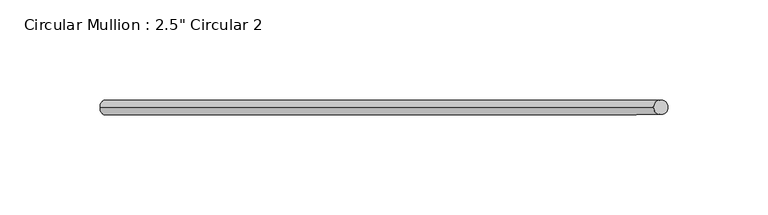
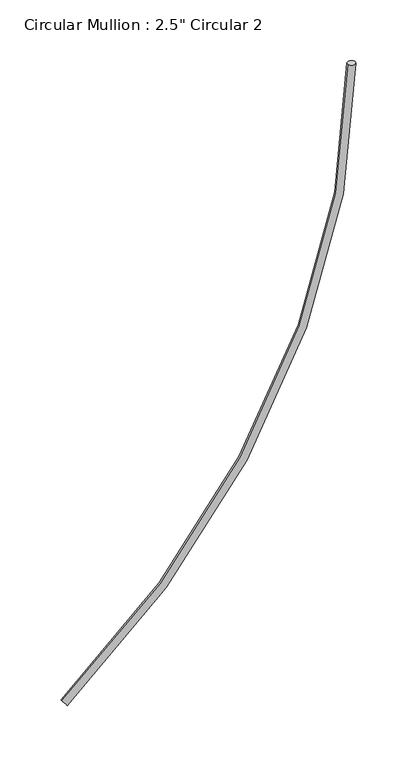
"""IFC4 building model written with IfcOpenShell, lengths in millimetres: member geometry."""

from ifc_helpers import new_model, si_unit, point, frame, origin, place, context, project, spatial, circle_curve, ellipse_curve, trimmed, source, transform, mapped, element, save
from ifc_brep_helpers import plane_surface, revolved_surface, advanced_brep


def member_6e035839(model_context):
    return source(origin(), model_context, "Body", "AdvancedBrep", [
        advanced_brep(
        [(-283.7434, 0.0, -553.0088), (-7.239, 0.0, 0.0), (0.0, 0.0, 0.0), (-279.4, 0.0, -558.8)],
        [
            (0, 1, circle_curve(frame((-698.5, 0.0, 0.0), z_axis=(0.0, -1.0, 0.0), x_axis=(1.0, 0.0, 0.0)), 691.261)),
            (1, 2, circle_curve(frame((-3.6195, 0.0, 0.0), z_axis=(0.0, 0.0, -1.0), x_axis=(1.0, 0.0, 0.0)), 3.6195)),
            (2, 3, circle_curve(frame((-698.5, 0.0, 0.0), z_axis=(0.0, 1.0, 0.0), x_axis=(1.0, 0.0, 0.0)), 698.5)),
            (3, 0, circle_curve(frame((-281.5717, 0.0, -555.9044), z_axis=(0.8000000000000037, 0.0, 0.5999999999999951), x_axis=(0.5999999999999951, 0.0, -0.8000000000000037)), 3.6195)),
            (2, 1, circle_curve(frame((-3.6195, 0.0, 0.0), z_axis=(0.0, 0.0, -1.0), x_axis=(1.0, 0.0, 0.0)), 3.6195)),
            (0, 3, circle_curve(frame((-281.5717, 0.0, -555.9044), z_axis=(0.8000000000000036, 0.0, 0.5999999999999952), x_axis=(0.5999999999999952, 0.0, -0.8000000000000036)), 3.6195)),
        ],
        [
            revolved_surface(trimmed(ellipse_curve(frame((-3.6195, 0.0, 0.0), z_axis=(0.0, 0.0, 1.0), x_axis=(1.0, 0.0, 0.0)), 3.6195, 3.6195), [point((0.0, 0.0, 0.0))], [point((-7.239, 0.0, 0.0))], True, "CARTESIAN"), (-698.5, 0.0, 0.0), (0.0, 1.0, 0.0)),
            revolved_surface(trimmed(ellipse_curve(frame((-3.6195, 0.0, 0.0), z_axis=(0.0, 0.0, 1.0), x_axis=(1.0, 0.0, 0.0)), 3.6195, 3.6195), [point((-7.239, 0.0, 0.0))], [point((0.0, 0.0, 0.0))], True, "CARTESIAN"), (-698.5, 0.0, 0.0), (0.0, 1.0, 0.0)),
            plane_surface(frame((-304.8, 0.0, 0.0), z_axis=(0.0, 0.0, 1.0), x_axis=(0.0, 1.0, 0.0))),
            plane_surface(frame((-96.52, 0.0, -802.64), z_axis=(-0.8000000000000039, 0.0, -0.5999999999999949), x_axis=(0.0, -1.0, 0.0))),
        ],
        [
            (0, [[1, 2, 3, 4]]),
            (1, [[-3, 5, -1, 6]]),
            (2, [[-2, -5]]),
            (3, [[-6, -4]]),
        ],
    ),
    ])


if __name__ == "__main__":
    model = new_model("IFC4")
    model_context = context("Model", 3, world=origin())
    ifc_project = project(units=[si_unit("LENGTHUNIT", "METRE", prefix="MILLI")], contexts=[model_context])
    site = spatial("IfcSite", under=ifc_project)
    building = spatial("IfcBuilding", under=site)
    placement = place(None, origin())
    member_shape = member_6e035839(model_context)
    element("IfcMember", 1, ObjectType="Circular Mullion : 2.5\" Circular 2", at=placement, inside=building, context=model_context, shape_type="MappedRepresentation", body=[
        mapped(member_shape, transform((0.0, 0.0, 0.0), x_axis=(1.0, 0.0, 0.0), y_axis=(0.0, 1.0, 0.0), z_axis=(0.0, 0.0, 1.0))),
    ])
    save(model, "model.ifc")

# Revit data of these elements
# Type "Circular Mullion : 2.5\" Circular 2"
#   built-in parameter 1007350 = 0.011875 (stored number, unit not read)
# Element 1 (IfcMember, "Circular Mullion : 2.5\" Circular 2")
#   Materials on its faces: "Aluminum"
# Materials
#   "Aluminum": class "Metal", colour RGB 247 247 247, transparency 0, Description = "Aluminum 6061", Cost = 0
